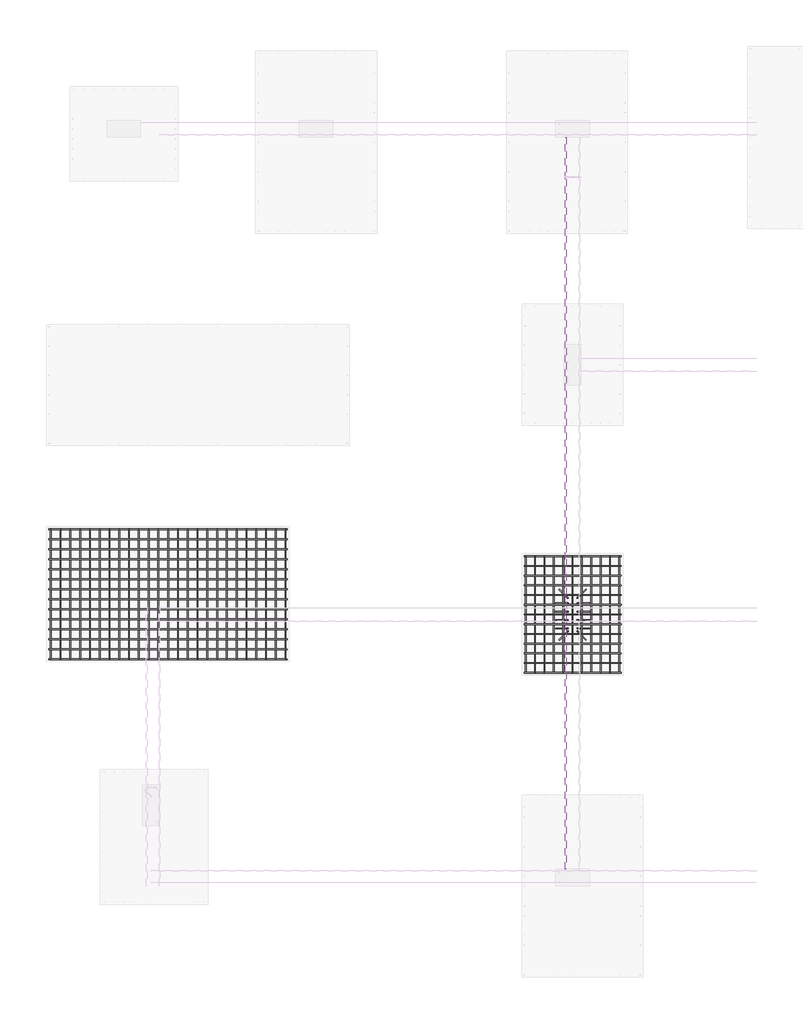
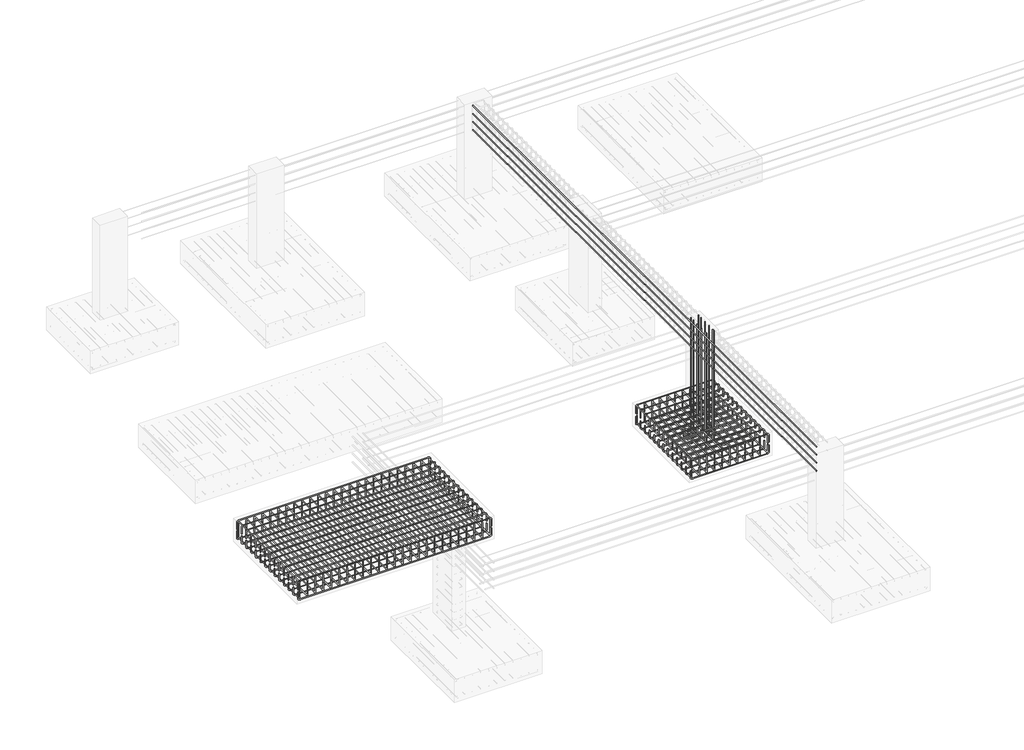
# One storey, part 3 of 16: 15 reinforcing bars.
"""IFC4 building model written with IfcOpenShell, lengths in millimetres."""

from ifc_helpers import new_model, si_unit, point, frame, origin, place, context, project, spatial, polyline, circle_curve, trimmed, segment, composite_curve, source, transform, mapped, element, save
from ifc_brep_helpers import swept_disk

model = new_model("IFC4")

# Units and contexts
model_context = context("Model", 3, world=origin())
ifc_project = project(units=[si_unit("LENGTHUNIT", "METRE", prefix="MILLI")], contexts=[model_context])

# Site, building, storey
site = spatial("IfcSite", under=ifc_project)
building = spatial("IfcBuilding", under=site)
storey = spatial("IfcBuildingStorey", under=building, Elevation=-1828.8)

# Reinforcing bars
placement = place(None, origin())
reinforcing_bar_shape = source(origin(), model_context, "Body", "SolidModel", [
    swept_disk(composite_curve([segment(polyline([(-8214.2725801, -1513.6888221, -2088.8), (-8214.2725801, -1513.6888221, -2212.8)]), True, "CONTINUOUS"), segment(trimmed(circle_curve(frame((-8244.2725801, -1513.6888221, -2212.8), z_axis=(0.0, 1.0, 0.0), x_axis=(30.0, 0.0, 0.0)), 30.0), [point((-8214.2725801, -1513.6888221, -2212.8))], [point((-8244.2725801, -1513.6888221, -2242.8))], True, "CARTESIAN"), True, "CONTINUOUS"), segment(polyline([(-8244.2725801, -1513.6888221, -2242.8), (-9612.2725801, -1513.6888221, -2242.8)]), True, "CONTINUOUS"), segment(trimmed(circle_curve(frame((-9612.2725801, -1513.6888221, -2212.8), z_axis=(0.0, 1.0, 0.0), x_axis=(0.0, 0.0, -30.0)), 30.0), [point((-9612.2725801, -1513.6888221, -2242.8))], [point((-9642.2725801, -1513.6888221, -2212.8))], True, "CARTESIAN"), True, "CONTINUOUS"), segment(polyline([(-9642.2725801, -1513.6888221, -2212.8), (-9642.2725801, -1513.6888221, -2088.8)]), True, "CONTINUOUS")], self_intersect=False), 6.0),
])
element("IfcReinforcingBar", 1, at=placement, inside=storey, context=model_context, shape_type="MappedRepresentation", body=[
    mapped(reinforcing_bar_shape, transform((0.0, 0.0, 0.0), x_axis=(1.0, 0.0, 0.0), y_axis=(0.0, 1.0, 0.0), z_axis=(0.0, 0.0, 1.0))),
    mapped(reinforcing_bar_shape, transform((0.0, -144.0, 0.0), x_axis=(1.0, 0.0, 0.0), y_axis=(0.0, 1.0, 0.0), z_axis=(0.0, 0.0, 1.0))),
    mapped(reinforcing_bar_shape, transform((0.0, -288.0, 0.0), x_axis=(1.0, 0.0, 0.0), y_axis=(0.0, 1.0, 0.0), z_axis=(0.0, 0.0, 1.0))),
    mapped(reinforcing_bar_shape, transform((0.0, -432.0, 0.0), x_axis=(1.0, 0.0, 0.0), y_axis=(0.0, 1.0, 0.0), z_axis=(0.0, 0.0, 1.0))),
    mapped(reinforcing_bar_shape, transform((0.0, -576.0, 0.0), x_axis=(1.0, 0.0, 0.0), y_axis=(0.0, 1.0, 0.0), z_axis=(0.0, 0.0, 1.0))),
    mapped(reinforcing_bar_shape, transform((0.0, -720.0, 0.0), x_axis=(1.0, 0.0, 0.0), y_axis=(0.0, 1.0, 0.0), z_axis=(0.0, 0.0, 1.0))),
    mapped(reinforcing_bar_shape, transform((0.0, -864.0, 0.0), x_axis=(1.0, 0.0, 0.0), y_axis=(0.0, 1.0, 0.0), z_axis=(0.0, 0.0, 1.0))),
    mapped(reinforcing_bar_shape, transform((0.0, -1008.0, 0.0), x_axis=(1.0, 0.0, 0.0), y_axis=(0.0, 1.0, 0.0), z_axis=(0.0, 0.0, 1.0))),
    mapped(reinforcing_bar_shape, transform((0.0, -1152.0, 0.0), x_axis=(1.0, 0.0, 0.0), y_axis=(0.0, 1.0, 0.0), z_axis=(0.0, 0.0, 1.0))),
    mapped(reinforcing_bar_shape, transform((0.0, -1296.0, 0.0), x_axis=(1.0, 0.0, 0.0), y_axis=(0.0, 1.0, 0.0), z_axis=(0.0, 0.0, 1.0))),
    mapped(reinforcing_bar_shape, transform((0.0, -1440.0, 0.0), x_axis=(1.0, 0.0, 0.0), y_axis=(0.0, 1.0, 0.0), z_axis=(0.0, 0.0, 1.0))),
    mapped(reinforcing_bar_shape, transform((0.0, -1584.0, 0.0), x_axis=(1.0, 0.0, 0.0), y_axis=(0.0, 1.0, 0.0), z_axis=(0.0, 0.0, 1.0))),
    mapped(reinforcing_bar_shape, transform((0.0, -1728.0, 0.0), x_axis=(1.0, 0.0, 0.0), y_axis=(0.0, 1.0, 0.0), z_axis=(0.0, 0.0, 1.0))),
])
reinforcing_bar_2_shape = source(origin(), model_context, "Body", "SolidModel", [
    swept_disk(composite_curve([segment(polyline([(-9642.2725801, -1513.6888221, -2018.8), (-9642.2725801, -1513.6888221, -1894.8)]), True, "CONTINUOUS"), segment(trimmed(circle_curve(frame((-9612.2725801, -1513.6888221, -1894.8), z_axis=(0.0, 1.0, 0.0), x_axis=(-30.0, 0.0, 0.0)), 30.0), [point((-9642.2725801, -1513.6888221, -1894.8))], [point((-9612.2725801, -1513.6888221, -1864.8))], True, "CARTESIAN"), True, "CONTINUOUS"), segment(polyline([(-9612.2725801, -1513.6888221, -1864.8), (-8244.2725801, -1513.6888221, -1864.8)]), True, "CONTINUOUS"), segment(trimmed(circle_curve(frame((-8244.2725801, -1513.6888221, -1894.8), z_axis=(0.0, 1.0, 0.0), x_axis=(0.0, 0.0, 30.0)), 30.0), [point((-8244.2725801, -1513.6888221, -1864.8))], [point((-8214.2725801, -1513.6888221, -1894.8))], True, "CARTESIAN"), True, "CONTINUOUS"), segment(polyline([(-8214.2725801, -1513.6888221, -1894.8), (-8214.2725801, -1513.6888221, -2018.8)]), True, "CONTINUOUS")], self_intersect=False), 6.0),
])
element("IfcReinforcingBar", 2, at=placement, inside=storey, context=model_context, shape_type="MappedRepresentation", body=[
    mapped(reinforcing_bar_2_shape, transform((0.0, 0.0, 0.0), x_axis=(1.0, 0.0, 0.0), y_axis=(0.0, 1.0, 0.0), z_axis=(0.0, 0.0, 1.0))),
    mapped(reinforcing_bar_2_shape, transform((0.0, -144.0, 0.0), x_axis=(1.0, 0.0, 0.0), y_axis=(0.0, 1.0, 0.0), z_axis=(0.0, 0.0, 1.0))),
    mapped(reinforcing_bar_2_shape, transform((0.0, -288.0, 0.0), x_axis=(1.0, 0.0, 0.0), y_axis=(0.0, 1.0, 0.0), z_axis=(0.0, 0.0, 1.0))),
    mapped(reinforcing_bar_2_shape, transform((0.0, -432.0, 0.0), x_axis=(1.0, 0.0, 0.0), y_axis=(0.0, 1.0, 0.0), z_axis=(0.0, 0.0, 1.0))),
    mapped(reinforcing_bar_2_shape, transform((0.0, -576.0, 0.0), x_axis=(1.0, 0.0, 0.0), y_axis=(0.0, 1.0, 0.0), z_axis=(0.0, 0.0, 1.0))),
    mapped(reinforcing_bar_2_shape, transform((0.0, -720.0, 0.0), x_axis=(1.0, 0.0, 0.0), y_axis=(0.0, 1.0, 0.0), z_axis=(0.0, 0.0, 1.0))),
    mapped(reinforcing_bar_2_shape, transform((0.0, -864.0, 0.0), x_axis=(1.0, 0.0, 0.0), y_axis=(0.0, 1.0, 0.0), z_axis=(0.0, 0.0, 1.0))),
    mapped(reinforcing_bar_2_shape, transform((0.0, -1008.0, 0.0), x_axis=(1.0, 0.0, 0.0), y_axis=(0.0, 1.0, 0.0), z_axis=(0.0, 0.0, 1.0))),
    mapped(reinforcing_bar_2_shape, transform((0.0, -1152.0, 0.0), x_axis=(1.0, 0.0, 0.0), y_axis=(0.0, 1.0, 0.0), z_axis=(0.0, 0.0, 1.0))),
    mapped(reinforcing_bar_2_shape, transform((0.0, -1296.0, 0.0), x_axis=(1.0, 0.0, 0.0), y_axis=(0.0, 1.0, 0.0), z_axis=(0.0, 0.0, 1.0))),
    mapped(reinforcing_bar_2_shape, transform((0.0, -1440.0, 0.0), x_axis=(1.0, 0.0, 0.0), y_axis=(0.0, 1.0, 0.0), z_axis=(0.0, 0.0, 1.0))),
    mapped(reinforcing_bar_2_shape, transform((0.0, -1584.0, 0.0), x_axis=(1.0, 0.0, 0.0), y_axis=(0.0, 1.0, 0.0), z_axis=(0.0, 0.0, 1.0))),
    mapped(reinforcing_bar_2_shape, transform((0.0, -1728.0, 0.0), x_axis=(1.0, 0.0, 0.0), y_axis=(0.0, 1.0, 0.0), z_axis=(0.0, 0.0, 1.0))),
])
reinforcing_bar_3_shape = source(origin(), model_context, "Body", "SolidModel", [
    swept_disk(composite_curve([segment(polyline([(-9625.0397909, -1513.6888221, -2072.0951729), (-9625.0397909, -1513.6888221, -2196.0951729)]), True, "CONTINUOUS"), segment(trimmed(circle_curve(frame((-9625.0397909, -1543.6888221, -2196.0951729), z_axis=(-1.0, 0.0, 0.0), x_axis=(0.0, 30.0, 0.0)), 30.0), [point((-9625.0397909, -1513.6888221, -2196.0951729))], [point((-9625.0397909, -1543.6888221, -2226.0951729))], True, "CARTESIAN"), True, "CONTINUOUS"), segment(polyline([(-9625.0397909, -1543.6888221, -2226.0951729), (-9625.0397909, -3211.6888221, -2226.0951729)]), True, "CONTINUOUS"), segment(trimmed(circle_curve(frame((-9625.0397909, -3211.6888221, -2196.0951729), z_axis=(-1.0, 0.0, 0.0), x_axis=(0.0, 0.0, -30.0)), 30.0), [point((-9625.0397909, -3211.6888221, -2226.0951729))], [point((-9625.0397909, -3241.6888221, -2196.0951729))], True, "CARTESIAN"), True, "CONTINUOUS"), segment(polyline([(-9625.0397909, -3241.6888221, -2196.0951729), (-9625.0397909, -3241.6888221, -2072.0951729)]), True, "CONTINUOUS")], self_intersect=False), 6.0),
])
element("IfcReinforcingBar", 3, at=placement, inside=storey, context=model_context, shape_type="MappedRepresentation", body=[
    mapped(reinforcing_bar_3_shape, transform((0.0, 0.0, 0.0), x_axis=(1.0, 0.0, 0.0), y_axis=(0.0, 1.0, 0.0), z_axis=(0.0, 0.0, 1.0))),
    mapped(reinforcing_bar_3_shape, transform((138.8820351, 0.0, 0.0), x_axis=(1.0, 0.0, 0.0), y_axis=(0.0, 1.0, 0.0), z_axis=(0.0, 0.0, 1.0))),
    mapped(reinforcing_bar_3_shape, transform((277.7640703, 0.0, 0.0), x_axis=(1.0, 0.0, 0.0), y_axis=(0.0, 1.0, 0.0), z_axis=(0.0, 0.0, 1.0))),
    mapped(reinforcing_bar_3_shape, transform((416.6461054, 0.0, 0.0), x_axis=(1.0, 0.0, 0.0), y_axis=(0.0, 1.0, 0.0), z_axis=(0.0, 0.0, 1.0))),
    mapped(reinforcing_bar_3_shape, transform((555.5281406, 0.0, 0.0), x_axis=(1.0, 0.0, 0.0), y_axis=(0.0, 1.0, 0.0), z_axis=(0.0, 0.0, 1.0))),
    mapped(reinforcing_bar_3_shape, transform((694.4101757, 0.0, 0.0), x_axis=(1.0, 0.0, 0.0), y_axis=(0.0, 1.0, 0.0), z_axis=(0.0, 0.0, 1.0))),
    mapped(reinforcing_bar_3_shape, transform((833.2922109, 0.0, 0.0), x_axis=(1.0, 0.0, 0.0), y_axis=(0.0, 1.0, 0.0), z_axis=(0.0, 0.0, 1.0))),
    mapped(reinforcing_bar_3_shape, transform((972.174246, 0.0, 0.0), x_axis=(1.0, 0.0, 0.0), y_axis=(0.0, 1.0, 0.0), z_axis=(0.0, 0.0, 1.0))),
    mapped(reinforcing_bar_3_shape, transform((1111.0562811, 0.0, 0.0), x_axis=(1.0, 0.0, 0.0), y_axis=(0.0, 1.0, 0.0), z_axis=(0.0, 0.0, 1.0))),
    mapped(reinforcing_bar_3_shape, transform((1249.9383163, 0.0, 0.0), x_axis=(1.0, 0.0, 0.0), y_axis=(0.0, 1.0, 0.0), z_axis=(0.0, 0.0, 1.0))),
    mapped(reinforcing_bar_3_shape, transform((1388.8203514, 0.0, 0.0), x_axis=(1.0, 0.0, 0.0), y_axis=(0.0, 1.0, 0.0), z_axis=(0.0, 0.0, 1.0))),
])
reinforcing_bar_4_shape = source(origin(), model_context, "Body", "SolidModel", [
    swept_disk(composite_curve([segment(polyline([(-8236.2194394, -1513.6888221, -2034.1277079), (-8236.2194394, -1513.6888221, -1910.1277079)]), True, "CONTINUOUS"), segment(trimmed(circle_curve(frame((-8236.2194394, -1543.6888221, -1910.1277079), z_axis=(1.0, 0.0, 0.0), x_axis=(0.0, 30.0, 0.0)), 30.0), [point((-8236.2194394, -1513.6888221, -1910.1277079))], [point((-8236.2194394, -1543.6888221, -1880.1277079))], True, "CARTESIAN"), True, "CONTINUOUS"), segment(polyline([(-8236.2194394, -1543.6888221, -1880.1277079), (-8236.2194394, -3211.6888221, -1880.1277079)]), True, "CONTINUOUS"), segment(trimmed(circle_curve(frame((-8236.2194394, -3211.6888221, -1910.1277079), z_axis=(1.0, 0.0, 0.0), x_axis=(0.0, 0.0, 30.0)), 30.0), [point((-8236.2194394, -3211.6888221, -1880.1277079))], [point((-8236.2194394, -3241.6888221, -1910.1277079))], True, "CARTESIAN"), True, "CONTINUOUS"), segment(polyline([(-8236.2194394, -3241.6888221, -1910.1277079), (-8236.2194394, -3241.6888221, -2034.1277079)]), True, "CONTINUOUS")], self_intersect=False), 6.0),
])
element("IfcReinforcingBar", 4, at=placement, inside=storey, context=model_context, shape_type="MappedRepresentation", body=[
    mapped(reinforcing_bar_4_shape, transform((0.0, 0.0, 0.0), x_axis=(1.0, 0.0, 0.0), y_axis=(0.0, 1.0, 0.0), z_axis=(0.0, 0.0, 1.0))),
    mapped(reinforcing_bar_4_shape, transform((-138.8820351, 0.0, 0.0), x_axis=(1.0, 0.0, 0.0), y_axis=(0.0, 1.0, 0.0), z_axis=(0.0, 0.0, 1.0))),
    mapped(reinforcing_bar_4_shape, transform((-277.7640703, 0.0, 0.0), x_axis=(1.0, 0.0, 0.0), y_axis=(0.0, 1.0, 0.0), z_axis=(0.0, 0.0, 1.0))),
    mapped(reinforcing_bar_4_shape, transform((-416.6461054, 0.0, 0.0), x_axis=(1.0, 0.0, 0.0), y_axis=(0.0, 1.0, 0.0), z_axis=(0.0, 0.0, 1.0))),
    mapped(reinforcing_bar_4_shape, transform((-555.5281406, 0.0, 0.0), x_axis=(1.0, 0.0, 0.0), y_axis=(0.0, 1.0, 0.0), z_axis=(0.0, 0.0, 1.0))),
    mapped(reinforcing_bar_4_shape, transform((-694.4101757, 0.0, 0.0), x_axis=(1.0, 0.0, 0.0), y_axis=(0.0, 1.0, 0.0), z_axis=(0.0, 0.0, 1.0))),
    mapped(reinforcing_bar_4_shape, transform((-833.2922109, 0.0, 0.0), x_axis=(1.0, 0.0, 0.0), y_axis=(0.0, 1.0, 0.0), z_axis=(0.0, 0.0, 1.0))),
    mapped(reinforcing_bar_4_shape, transform((-972.174246, 0.0, 0.0), x_axis=(1.0, 0.0, 0.0), y_axis=(0.0, 1.0, 0.0), z_axis=(0.0, 0.0, 1.0))),
    mapped(reinforcing_bar_4_shape, transform((-1111.0562811, 0.0, 0.0), x_axis=(1.0, 0.0, 0.0), y_axis=(0.0, 1.0, 0.0), z_axis=(0.0, 0.0, 1.0))),
    mapped(reinforcing_bar_4_shape, transform((-1249.9383163, 0.0, 0.0), x_axis=(1.0, 0.0, 0.0), y_axis=(0.0, 1.0, 0.0), z_axis=(0.0, 0.0, 1.0))),
    mapped(reinforcing_bar_4_shape, transform((-1388.8203514, 0.0, 0.0), x_axis=(1.0, 0.0, 0.0), y_axis=(0.0, 1.0, 0.0), z_axis=(0.0, 0.0, 1.0))),
])
reinforcing_bar_5_shape = source(origin(), model_context, "Body", "SolidModel", [
    swept_disk(composite_curve([segment(polyline([(-13164.3116599, -1115.1308991, -2072.7646888), (-13164.3116599, -1115.1308991, -2196.7646888)]), True, "CONTINUOUS"), segment(trimmed(circle_curve(frame((-13194.3116599, -1115.1308991, -2196.7646888), z_axis=(0.0, 1.0, 0.0), x_axis=(30.0, 0.0, 0.0)), 30.0), [point((-13164.3116599, -1115.1308991, -2196.7646888))], [point((-13194.3116599, -1115.1308991, -2226.7646888))], True, "CARTESIAN"), True, "CONTINUOUS"), segment(polyline([(-13194.3116599, -1115.1308991, -2226.7646888), (-16662.3116599, -1115.1308991, -2226.7646888)]), True, "CONTINUOUS"), segment(trimmed(circle_curve(frame((-16662.3116599, -1115.1308991, -2196.7646888), z_axis=(0.0, 1.0, 0.0), x_axis=(0.0, 0.0, -30.0)), 30.0), [point((-16662.3116599, -1115.1308991, -2226.7646888))], [point((-16692.3116599, -1115.1308991, -2196.7646888))], True, "CARTESIAN"), True, "CONTINUOUS"), segment(polyline([(-16692.3116599, -1115.1308991, -2196.7646888), (-16692.3116599, -1115.1308991, -2072.7646888)]), True, "CONTINUOUS")], self_intersect=False), 6.0),
])
element("IfcReinforcingBar", 5, at=placement, inside=storey, context=model_context, shape_type="MappedRepresentation", body=[
    mapped(reinforcing_bar_5_shape, transform((0.0, 0.0, 0.0), x_axis=(1.0, 0.0, 0.0), y_axis=(0.0, 1.0, 0.0), z_axis=(0.0, 0.0, 1.0))),
    mapped(reinforcing_bar_5_shape, transform((0.0, -148.3076923, 0.0), x_axis=(1.0, 0.0, 0.0), y_axis=(0.0, 1.0, 0.0), z_axis=(0.0, 0.0, 1.0))),
    mapped(reinforcing_bar_5_shape, transform((0.0, -296.6153846, 0.0), x_axis=(1.0, 0.0, 0.0), y_axis=(0.0, 1.0, 0.0), z_axis=(0.0, 0.0, 1.0))),
    mapped(reinforcing_bar_5_shape, transform((0.0, -444.9230769, 0.0), x_axis=(1.0, 0.0, 0.0), y_axis=(0.0, 1.0, 0.0), z_axis=(0.0, 0.0, 1.0))),
    mapped(reinforcing_bar_5_shape, transform((0.0, -593.2307692, 0.0), x_axis=(1.0, 0.0, 0.0), y_axis=(0.0, 1.0, 0.0), z_axis=(0.0, 0.0, 1.0))),
    mapped(reinforcing_bar_5_shape, transform((0.0, -741.5384615, 0.0), x_axis=(1.0, 0.0, 0.0), y_axis=(0.0, 1.0, 0.0), z_axis=(0.0, 0.0, 1.0))),
    mapped(reinforcing_bar_5_shape, transform((0.0, -889.8461538, 0.0), x_axis=(1.0, 0.0, 0.0), y_axis=(0.0, 1.0, 0.0), z_axis=(0.0, 0.0, 1.0))),
    mapped(reinforcing_bar_5_shape, transform((0.0, -1038.1538462, 0.0), x_axis=(1.0, 0.0, 0.0), y_axis=(0.0, 1.0, 0.0), z_axis=(0.0, 0.0, 1.0))),
    mapped(reinforcing_bar_5_shape, transform((0.0, -1186.4615385, 0.0), x_axis=(1.0, 0.0, 0.0), y_axis=(0.0, 1.0, 0.0), z_axis=(0.0, 0.0, 1.0))),
    mapped(reinforcing_bar_5_shape, transform((0.0, -1334.7692308, 0.0), x_axis=(1.0, 0.0, 0.0), y_axis=(0.0, 1.0, 0.0), z_axis=(0.0, 0.0, 1.0))),
    mapped(reinforcing_bar_5_shape, transform((0.0, -1483.0769231, 0.0), x_axis=(1.0, 0.0, 0.0), y_axis=(0.0, 1.0, 0.0), z_axis=(0.0, 0.0, 1.0))),
    mapped(reinforcing_bar_5_shape, transform((0.0, -1631.3846154, 0.0), x_axis=(1.0, 0.0, 0.0), y_axis=(0.0, 1.0, 0.0), z_axis=(0.0, 0.0, 1.0))),
    mapped(reinforcing_bar_5_shape, transform((0.0, -1779.6923077, 0.0), x_axis=(1.0, 0.0, 0.0), y_axis=(0.0, 1.0, 0.0), z_axis=(0.0, 0.0, 1.0))),
    mapped(reinforcing_bar_5_shape, transform((0.0, -1928.0, 0.0), x_axis=(1.0, 0.0, 0.0), y_axis=(0.0, 1.0, 0.0), z_axis=(0.0, 0.0, 1.0))),
])
reinforcing_bar_6_shape = source(origin(), model_context, "Body", "SolidModel", [
    swept_disk(composite_curve([segment(polyline([(-16692.3116599, -1115.1308991, -2026.8886474), (-16692.3116599, -1115.1308991, -1902.8886474)]), True, "CONTINUOUS"), segment(trimmed(circle_curve(frame((-16662.3116599, -1115.1308991, -1902.8886474), z_axis=(0.0, 1.0, 0.0), x_axis=(-30.0, 0.0, 0.0)), 30.0), [point((-16692.3116599, -1115.1308991, -1902.8886474))], [point((-16662.3116599, -1115.1308991, -1872.8886474))], True, "CARTESIAN"), True, "CONTINUOUS"), segment(polyline([(-16662.3116599, -1115.1308991, -1872.8886474), (-13194.3116599, -1115.1308991, -1872.8886474)]), True, "CONTINUOUS"), segment(trimmed(circle_curve(frame((-13194.3116599, -1115.1308991, -1902.8886474), z_axis=(0.0, 1.0, 0.0), x_axis=(0.0, 0.0, 30.0)), 30.0), [point((-13194.3116599, -1115.1308991, -1872.8886474))], [point((-13164.3116599, -1115.1308991, -1902.8886474))], True, "CARTESIAN"), True, "CONTINUOUS"), segment(polyline([(-13164.3116599, -1115.1308991, -1902.8886474), (-13164.3116599, -1115.1308991, -2026.8886474)]), True, "CONTINUOUS")], self_intersect=False), 6.0),
])
element("IfcReinforcingBar", 6, at=placement, inside=storey, context=model_context, shape_type="MappedRepresentation", body=[
    mapped(reinforcing_bar_6_shape, transform((0.0, 0.0, 0.0), x_axis=(1.0, 0.0, 0.0), y_axis=(0.0, 1.0, 0.0), z_axis=(0.0, 0.0, 1.0))),
    mapped(reinforcing_bar_6_shape, transform((0.0, -148.3076923, 0.0), x_axis=(1.0, 0.0, 0.0), y_axis=(0.0, 1.0, 0.0), z_axis=(0.0, 0.0, 1.0))),
    mapped(reinforcing_bar_6_shape, transform((0.0, -296.6153846, 0.0), x_axis=(1.0, 0.0, 0.0), y_axis=(0.0, 1.0, 0.0), z_axis=(0.0, 0.0, 1.0))),
    mapped(reinforcing_bar_6_shape, transform((0.0, -444.9230769, 0.0), x_axis=(1.0, 0.0, 0.0), y_axis=(0.0, 1.0, 0.0), z_axis=(0.0, 0.0, 1.0))),
    mapped(reinforcing_bar_6_shape, transform((0.0, -593.2307692, 0.0), x_axis=(1.0, 0.0, 0.0), y_axis=(0.0, 1.0, 0.0), z_axis=(0.0, 0.0, 1.0))),
    mapped(reinforcing_bar_6_shape, transform((0.0, -741.5384615, 0.0), x_axis=(1.0, 0.0, 0.0), y_axis=(0.0, 1.0, 0.0), z_axis=(0.0, 0.0, 1.0))),
    mapped(reinforcing_bar_6_shape, transform((0.0, -889.8461538, 0.0), x_axis=(1.0, 0.0, 0.0), y_axis=(0.0, 1.0, 0.0), z_axis=(0.0, 0.0, 1.0))),
    mapped(reinforcing_bar_6_shape, transform((0.0, -1038.1538462, 0.0), x_axis=(1.0, 0.0, 0.0), y_axis=(0.0, 1.0, 0.0), z_axis=(0.0, 0.0, 1.0))),
    mapped(reinforcing_bar_6_shape, transform((0.0, -1186.4615385, 0.0), x_axis=(1.0, 0.0, 0.0), y_axis=(0.0, 1.0, 0.0), z_axis=(0.0, 0.0, 1.0))),
    mapped(reinforcing_bar_6_shape, transform((0.0, -1334.7692308, 0.0), x_axis=(1.0, 0.0, 0.0), y_axis=(0.0, 1.0, 0.0), z_axis=(0.0, 0.0, 1.0))),
    mapped(reinforcing_bar_6_shape, transform((0.0, -1483.0769231, 0.0), x_axis=(1.0, 0.0, 0.0), y_axis=(0.0, 1.0, 0.0), z_axis=(0.0, 0.0, 1.0))),
    mapped(reinforcing_bar_6_shape, transform((0.0, -1631.3846154, 0.0), x_axis=(1.0, 0.0, 0.0), y_axis=(0.0, 1.0, 0.0), z_axis=(0.0, 0.0, 1.0))),
    mapped(reinforcing_bar_6_shape, transform((0.0, -1779.6923077, 0.0), x_axis=(1.0, 0.0, 0.0), y_axis=(0.0, 1.0, 0.0), z_axis=(0.0, 0.0, 1.0))),
    mapped(reinforcing_bar_6_shape, transform((0.0, -1928.0, 0.0), x_axis=(1.0, 0.0, 0.0), y_axis=(0.0, 1.0, 0.0), z_axis=(0.0, 0.0, 1.0))),
])
reinforcing_bar_7_shape = source(origin(), model_context, "Body", "SolidModel", [
    swept_disk(composite_curve([segment(polyline([(-16665.3962792, -1115.1308991, -2055.302566), (-16665.3962792, -1115.1308991, -2179.302566)]), True, "CONTINUOUS"), segment(trimmed(circle_curve(frame((-16665.3962792, -1145.1308991, -2179.302566), z_axis=(-1.0, 0.0, 0.0), x_axis=(0.0, 30.0, 0.0)), 30.0), [point((-16665.3962792, -1115.1308991, -2179.302566))], [point((-16665.3962792, -1145.1308991, -2209.302566))], True, "CARTESIAN"), True, "CONTINUOUS"), segment(polyline([(-16665.3962792, -1145.1308991, -2209.302566), (-16665.3962792, -3013.1308991, -2209.302566)]), True, "CONTINUOUS"), segment(trimmed(circle_curve(frame((-16665.3962792, -3013.1308991, -2179.302566), z_axis=(-1.0, 0.0, 0.0), x_axis=(0.0, 0.0, -30.0)), 30.0), [point((-16665.3962792, -3013.1308991, -2209.302566))], [point((-16665.3962792, -3043.1308991, -2179.302566))], True, "CARTESIAN"), True, "CONTINUOUS"), segment(polyline([(-16665.3962792, -3043.1308991, -2179.302566), (-16665.3962792, -3043.1308991, -2055.302566)]), True, "CONTINUOUS")], self_intersect=False), 6.0),
])
element("IfcReinforcingBar", 7, at=placement, inside=storey, context=model_context, shape_type="MappedRepresentation", body=[
    mapped(reinforcing_bar_7_shape, transform((0.0, 0.0, 0.0), x_axis=(1.0, 0.0, 0.0), y_axis=(0.0, 1.0, 0.0), z_axis=(0.0, 0.0, 1.0))),
    mapped(reinforcing_bar_7_shape, transform((145.0375224, 0.0, 0.0), x_axis=(1.0, 0.0, 0.0), y_axis=(0.0, 1.0, 0.0), z_axis=(0.0, 0.0, 1.0))),
    mapped(reinforcing_bar_7_shape, transform((290.0750448, 0.0, 0.0), x_axis=(1.0, 0.0, 0.0), y_axis=(0.0, 1.0, 0.0), z_axis=(0.0, 0.0, 1.0))),
    mapped(reinforcing_bar_7_shape, transform((435.1125672, 0.0, 0.0), x_axis=(1.0, 0.0, 0.0), y_axis=(0.0, 1.0, 0.0), z_axis=(0.0, 0.0, 1.0))),
    mapped(reinforcing_bar_7_shape, transform((580.1500896, 0.0, 0.0), x_axis=(1.0, 0.0, 0.0), y_axis=(0.0, 1.0, 0.0), z_axis=(0.0, 0.0, 1.0))),
    mapped(reinforcing_bar_7_shape, transform((725.187612, 0.0, 0.0), x_axis=(1.0, 0.0, 0.0), y_axis=(0.0, 1.0, 0.0), z_axis=(0.0, 0.0, 1.0))),
    mapped(reinforcing_bar_7_shape, transform((870.2251345, 0.0, 0.0), x_axis=(1.0, 0.0, 0.0), y_axis=(0.0, 1.0, 0.0), z_axis=(0.0, 0.0, 1.0))),
    mapped(reinforcing_bar_7_shape, transform((1015.2626569, 0.0, 0.0), x_axis=(1.0, 0.0, 0.0), y_axis=(0.0, 1.0, 0.0), z_axis=(0.0, 0.0, 1.0))),
    mapped(reinforcing_bar_7_shape, transform((1160.3001793, 0.0, 0.0), x_axis=(1.0, 0.0, 0.0), y_axis=(0.0, 1.0, 0.0), z_axis=(0.0, 0.0, 1.0))),
    mapped(reinforcing_bar_7_shape, transform((1305.3377017, 0.0, 0.0), x_axis=(1.0, 0.0, 0.0), y_axis=(0.0, 1.0, 0.0), z_axis=(0.0, 0.0, 1.0))),
    mapped(reinforcing_bar_7_shape, transform((1450.3752241, 0.0, 0.0), x_axis=(1.0, 0.0, 0.0), y_axis=(0.0, 1.0, 0.0), z_axis=(0.0, 0.0, 1.0))),
    mapped(reinforcing_bar_7_shape, transform((1595.4127465, 0.0, 0.0), x_axis=(1.0, 0.0, 0.0), y_axis=(0.0, 1.0, 0.0), z_axis=(0.0, 0.0, 1.0))),
    mapped(reinforcing_bar_7_shape, transform((1740.4502689, 0.0, 0.0), x_axis=(1.0, 0.0, 0.0), y_axis=(0.0, 1.0, 0.0), z_axis=(0.0, 0.0, 1.0))),
    mapped(reinforcing_bar_7_shape, transform((1885.4877913, 0.0, 0.0), x_axis=(1.0, 0.0, 0.0), y_axis=(0.0, 1.0, 0.0), z_axis=(0.0, 0.0, 1.0))),
    mapped(reinforcing_bar_7_shape, transform((2030.5253137, 0.0, 0.0), x_axis=(1.0, 0.0, 0.0), y_axis=(0.0, 1.0, 0.0), z_axis=(0.0, 0.0, 1.0))),
    mapped(reinforcing_bar_7_shape, transform((2175.5628361, 0.0, 0.0), x_axis=(1.0, 0.0, 0.0), y_axis=(0.0, 1.0, 0.0), z_axis=(0.0, 0.0, 1.0))),
    mapped(reinforcing_bar_7_shape, transform((2320.6003586, 0.0, 0.0), x_axis=(1.0, 0.0, 0.0), y_axis=(0.0, 1.0, 0.0), z_axis=(0.0, 0.0, 1.0))),
    mapped(reinforcing_bar_7_shape, transform((2465.637881, 0.0, 0.0), x_axis=(1.0, 0.0, 0.0), y_axis=(0.0, 1.0, 0.0), z_axis=(0.0, 0.0, 1.0))),
    mapped(reinforcing_bar_7_shape, transform((2610.6754034, 0.0, 0.0), x_axis=(1.0, 0.0, 0.0), y_axis=(0.0, 1.0, 0.0), z_axis=(0.0, 0.0, 1.0))),
    mapped(reinforcing_bar_7_shape, transform((2755.7129258, 0.0, 0.0), x_axis=(1.0, 0.0, 0.0), y_axis=(0.0, 1.0, 0.0), z_axis=(0.0, 0.0, 1.0))),
    mapped(reinforcing_bar_7_shape, transform((2900.7504482, 0.0, 0.0), x_axis=(1.0, 0.0, 0.0), y_axis=(0.0, 1.0, 0.0), z_axis=(0.0, 0.0, 1.0))),
    mapped(reinforcing_bar_7_shape, transform((3045.7879706, 0.0, 0.0), x_axis=(1.0, 0.0, 0.0), y_axis=(0.0, 1.0, 0.0), z_axis=(0.0, 0.0, 1.0))),
    mapped(reinforcing_bar_7_shape, transform((3190.825493, 0.0, 0.0), x_axis=(1.0, 0.0, 0.0), y_axis=(0.0, 1.0, 0.0), z_axis=(0.0, 0.0, 1.0))),
    mapped(reinforcing_bar_7_shape, transform((3335.8630154, 0.0, 0.0), x_axis=(1.0, 0.0, 0.0), y_axis=(0.0, 1.0, 0.0), z_axis=(0.0, 0.0, 1.0))),
    mapped(reinforcing_bar_7_shape, transform((3480.9005378, 0.0, 0.0), x_axis=(1.0, 0.0, 0.0), y_axis=(0.0, 1.0, 0.0), z_axis=(0.0, 0.0, 1.0))),
])
reinforcing_bar_8_shape = source(origin(), model_context, "Body", "SolidModel", [
    swept_disk(composite_curve([segment(polyline([(-13184.4957413, -1115.1308991, -2042.2263024), (-13184.4957413, -1115.1308991, -1918.2263024)]), True, "CONTINUOUS"), segment(trimmed(circle_curve(frame((-13184.4957413, -1145.1308991, -1918.2263024), z_axis=(1.0, 0.0, 0.0), x_axis=(0.0, 30.0, 0.0)), 30.0), [point((-13184.4957413, -1115.1308991, -1918.2263024))], [point((-13184.4957413, -1145.1308991, -1888.2263024))], True, "CARTESIAN"), True, "CONTINUOUS"), segment(polyline([(-13184.4957413, -1145.1308991, -1888.2263024), (-13184.4957413, -3013.1308991, -1888.2263024)]), True, "CONTINUOUS"), segment(trimmed(circle_curve(frame((-13184.4957413, -3013.1308991, -1918.2263024), z_axis=(1.0, 0.0, 0.0), x_axis=(0.0, 0.0, 30.0)), 30.0), [point((-13184.4957413, -3013.1308991, -1888.2263024))], [point((-13184.4957413, -3043.1308991, -1918.2263024))], True, "CARTESIAN"), True, "CONTINUOUS"), segment(polyline([(-13184.4957413, -3043.1308991, -1918.2263024), (-13184.4957413, -3043.1308991, -2042.2263024)]), True, "CONTINUOUS")], self_intersect=False), 6.0),
])
element("IfcReinforcingBar", 8, at=placement, inside=storey, context=model_context, shape_type="MappedRepresentation", body=[
    mapped(reinforcing_bar_8_shape, transform((0.0, 0.0, 0.0), x_axis=(1.0, 0.0, 0.0), y_axis=(0.0, 1.0, 0.0), z_axis=(0.0, 0.0, 1.0))),
    mapped(reinforcing_bar_8_shape, transform((-145.0375224, 0.0, 0.0), x_axis=(1.0, 0.0, 0.0), y_axis=(0.0, 1.0, 0.0), z_axis=(0.0, 0.0, 1.0))),
    mapped(reinforcing_bar_8_shape, transform((-290.0750448, 0.0, 0.0), x_axis=(1.0, 0.0, 0.0), y_axis=(0.0, 1.0, 0.0), z_axis=(0.0, 0.0, 1.0))),
    mapped(reinforcing_bar_8_shape, transform((-435.1125672, 0.0, 0.0), x_axis=(1.0, 0.0, 0.0), y_axis=(0.0, 1.0, 0.0), z_axis=(0.0, 0.0, 1.0))),
    mapped(reinforcing_bar_8_shape, transform((-580.1500896, 0.0, 0.0), x_axis=(1.0, 0.0, 0.0), y_axis=(0.0, 1.0, 0.0), z_axis=(0.0, 0.0, 1.0))),
    mapped(reinforcing_bar_8_shape, transform((-725.187612, 0.0, 0.0), x_axis=(1.0, 0.0, 0.0), y_axis=(0.0, 1.0, 0.0), z_axis=(0.0, 0.0, 1.0))),
    mapped(reinforcing_bar_8_shape, transform((-870.2251345, 0.0, 0.0), x_axis=(1.0, 0.0, 0.0), y_axis=(0.0, 1.0, 0.0), z_axis=(0.0, 0.0, 1.0))),
    mapped(reinforcing_bar_8_shape, transform((-1015.2626569, 0.0, 0.0), x_axis=(1.0, 0.0, 0.0), y_axis=(0.0, 1.0, 0.0), z_axis=(0.0, 0.0, 1.0))),
    mapped(reinforcing_bar_8_shape, transform((-1160.3001793, 0.0, 0.0), x_axis=(1.0, 0.0, 0.0), y_axis=(0.0, 1.0, 0.0), z_axis=(0.0, 0.0, 1.0))),
    mapped(reinforcing_bar_8_shape, transform((-1305.3377017, 0.0, 0.0), x_axis=(1.0, 0.0, 0.0), y_axis=(0.0, 1.0, 0.0), z_axis=(0.0, 0.0, 1.0))),
    mapped(reinforcing_bar_8_shape, transform((-1450.3752241, 0.0, 0.0), x_axis=(1.0, 0.0, 0.0), y_axis=(0.0, 1.0, 0.0), z_axis=(0.0, 0.0, 1.0))),
    mapped(reinforcing_bar_8_shape, transform((-1595.4127465, 0.0, 0.0), x_axis=(1.0, 0.0, 0.0), y_axis=(0.0, 1.0, 0.0), z_axis=(0.0, 0.0, 1.0))),
    mapped(reinforcing_bar_8_shape, transform((-1740.4502689, 0.0, 0.0), x_axis=(1.0, 0.0, 0.0), y_axis=(0.0, 1.0, 0.0), z_axis=(0.0, 0.0, 1.0))),
    mapped(reinforcing_bar_8_shape, transform((-1885.4877913, 0.0, 0.0), x_axis=(1.0, 0.0, 0.0), y_axis=(0.0, 1.0, 0.0), z_axis=(0.0, 0.0, 1.0))),
    mapped(reinforcing_bar_8_shape, transform((-2030.5253137, 0.0, 0.0), x_axis=(1.0, 0.0, 0.0), y_axis=(0.0, 1.0, 0.0), z_axis=(0.0, 0.0, 1.0))),
    mapped(reinforcing_bar_8_shape, transform((-2175.5628361, 0.0, 0.0), x_axis=(1.0, 0.0, 0.0), y_axis=(0.0, 1.0, 0.0), z_axis=(0.0, 0.0, 1.0))),
    mapped(reinforcing_bar_8_shape, transform((-2320.6003586, 0.0, 0.0), x_axis=(1.0, 0.0, 0.0), y_axis=(0.0, 1.0, 0.0), z_axis=(0.0, 0.0, 1.0))),
    mapped(reinforcing_bar_8_shape, transform((-2465.637881, 0.0, 0.0), x_axis=(1.0, 0.0, 0.0), y_axis=(0.0, 1.0, 0.0), z_axis=(0.0, 0.0, 1.0))),
    mapped(reinforcing_bar_8_shape, transform((-2610.6754034, 0.0, 0.0), x_axis=(1.0, 0.0, 0.0), y_axis=(0.0, 1.0, 0.0), z_axis=(0.0, 0.0, 1.0))),
    mapped(reinforcing_bar_8_shape, transform((-2755.7129258, 0.0, 0.0), x_axis=(1.0, 0.0, 0.0), y_axis=(0.0, 1.0, 0.0), z_axis=(0.0, 0.0, 1.0))),
    mapped(reinforcing_bar_8_shape, transform((-2900.7504482, 0.0, 0.0), x_axis=(1.0, 0.0, 0.0), y_axis=(0.0, 1.0, 0.0), z_axis=(0.0, 0.0, 1.0))),
    mapped(reinforcing_bar_8_shape, transform((-3045.7879706, 0.0, 0.0), x_axis=(1.0, 0.0, 0.0), y_axis=(0.0, 1.0, 0.0), z_axis=(0.0, 0.0, 1.0))),
    mapped(reinforcing_bar_8_shape, transform((-3190.825493, 0.0, 0.0), x_axis=(1.0, 0.0, 0.0), y_axis=(0.0, 1.0, 0.0), z_axis=(0.0, 0.0, 1.0))),
    mapped(reinforcing_bar_8_shape, transform((-3335.8630154, 0.0, 0.0), x_axis=(1.0, 0.0, 0.0), y_axis=(0.0, 1.0, 0.0), z_axis=(0.0, 0.0, 1.0))),
    mapped(reinforcing_bar_8_shape, transform((-3480.9005378, 0.0, 0.0), x_axis=(1.0, 0.0, 0.0), y_axis=(0.0, 1.0, 0.0), z_axis=(0.0, 0.0, 1.0))),
])
reinforcing_bar_9_shape = source(origin(), model_context, "Body", "SolidModel", [
    swept_disk(composite_curve([segment(polyline([(-8858.2317051, -2212.2776925, -30.0), (-8858.2317051, -2212.2776925, -2158.8)]), True, "CONTINUOUS"), segment(trimmed(circle_curve(frame((-8828.2317051, -2212.2776925, -2158.8), z_axis=(0.0, -1.0, 0.0), x_axis=(-30.0, 0.0, 0.0)), 30.0), [point((-8858.2317051, -2212.2776925, -2158.8))], [point((-8828.2317051, -2212.2776925, -2188.8))], True, "CARTESIAN"), True, "CONTINUOUS"), segment(polyline([(-8828.2317051, -2212.2776925, -2188.8), (-8675.8458602, -2212.2776925, -2188.8)]), True, "CONTINUOUS")], self_intersect=False), 6.0),
])
element("IfcReinforcingBar", 9, at=placement, inside=storey, context=model_context, shape_type="MappedRepresentation", body=[
    mapped(reinforcing_bar_9_shape, transform((0.0, 0.0, 0.0), x_axis=(1.0, 0.0, 0.0), y_axis=(0.0, 1.0, 0.0), z_axis=(0.0, 0.0, 1.0))),
    mapped(reinforcing_bar_9_shape, transform((0.0, -123.8384715, 0.0), x_axis=(1.0, 0.0, 0.0), y_axis=(0.0, 1.0, 0.0), z_axis=(0.0, 0.0, 1.0))),
    mapped(reinforcing_bar_9_shape, transform((0.0, -247.676943, 0.0), x_axis=(1.0, 0.0, 0.0), y_axis=(0.0, 1.0, 0.0), z_axis=(0.0, 0.0, 1.0))),
    mapped(reinforcing_bar_9_shape, transform((0.0, -371.5154145, 0.0), x_axis=(1.0, 0.0, 0.0), y_axis=(0.0, 1.0, 0.0), z_axis=(0.0, 0.0, 1.0))),
])
element("IfcReinforcingBar", 10, at=placement, inside=storey, context=model_context, shape_type="SolidModel", body=[
    swept_disk(composite_curve([segment(polyline([(-8998.3134551, -2134.0900242, -30.0), (-8998.3134551, -2134.0900242, -2158.8)]), True, "CONTINUOUS"), segment(trimmed(circle_curve(frame((-9019.5266585, -2112.8768207, -2158.8), z_axis=(0.7071067811865435, 0.7071067811865517, 0.0), x_axis=(21.213203400000566, -21.213203499999963, 0.0)), 30.0), [point((-8998.3134551, -2134.0900242, -2158.8))], [point((-9019.5266585, -2112.8768207, -2188.8))], True, "CARTESIAN"), True, "CONTINUOUS"), segment(polyline([(-9019.5266585, -2112.8768207, -2188.8), (-9127.2797228, -2005.1237565, -2188.8)]), True, "CONTINUOUS")], self_intersect=False), 6.0),
])
element("IfcReinforcingBar", 11, at=placement, inside=storey, context=model_context, shape_type="SolidModel", body=[
    swept_disk(composite_curve([segment(polyline([(-8858.2317051, -2624.1717741, -30.0), (-8858.2317051, -2624.1717741, -2158.8)]), True, "CONTINUOUS"), segment(trimmed(circle_curve(frame((-8837.0185017, -2645.3849776, -2158.8), z_axis=(-0.7071067811865435, -0.7071067811865517, 0.0), x_axis=(-21.213203400000566, 21.213203499999963, 0.0)), 30.0), [point((-8858.2317051, -2624.1717741, -2158.8))], [point((-8837.0185017, -2645.3849776, -2188.8))], True, "CARTESIAN"), True, "CONTINUOUS"), segment(polyline([(-8837.0185017, -2645.3849776, -2188.8), (-8729.2654374, -2753.1380418, -2188.8)]), True, "CONTINUOUS")], self_intersect=False), 6.0),
])
element("IfcReinforcingBar", 12, at=placement, inside=storey, context=model_context, shape_type="SolidModel", body=[
    swept_disk(composite_curve([segment(polyline([(-8998.3134551, -2624.1717741, -30.0), (-8998.3134551, -2624.1717741, -2158.8)]), True, "CONTINUOUS"), segment(trimmed(circle_curve(frame((-9019.5266585, -2645.3849776, -2158.8), z_axis=(-0.7071067811865435, 0.7071067811865516, 0.0), x_axis=(21.213203400000566, 21.213203499999963, 0.0)), 30.0), [point((-8998.3134551, -2624.1717741, -2158.8))], [point((-9019.5266585, -2645.3849776, -2188.8))], True, "CARTESIAN"), True, "CONTINUOUS"), segment(polyline([(-9019.5266585, -2645.3849776, -2188.8), (-9127.2797228, -2753.1380418, -2188.8)]), True, "CONTINUOUS")], self_intersect=False), 6.0),
])
element("IfcReinforcingBar", 13, at=placement, inside=storey, context=model_context, shape_type="SolidModel", body=[
    swept_disk(composite_curve([segment(polyline([(-8858.2317051, -2134.0900242, -30.0), (-8858.2317051, -2134.0900242, -2158.8)]), True, "CONTINUOUS"), segment(trimmed(circle_curve(frame((-8837.0185017, -2112.8768207, -2158.8), z_axis=(0.7071067811865434, -0.7071067811865518, 0.0), x_axis=(-21.213203400000566, -21.213203499999963, 0.0)), 30.0), [point((-8858.2317051, -2134.0900242, -2158.8))], [point((-8837.0185017, -2112.8768207, -2188.8))], True, "CARTESIAN"), True, "CONTINUOUS"), segment(polyline([(-8837.0185017, -2112.8768207, -2188.8), (-8729.2654374, -2005.1237565, -2188.8)]), True, "CONTINUOUS")], self_intersect=False), 6.0),
])
reinforcing_bar_10_shape = source(origin(), model_context, "Body", "SolidModel", [
    swept_disk(composite_curve([segment(polyline([(-8998.3134551, -2212.2776925, -30.0), (-8998.3134551, -2212.2776925, -2158.8)]), True, "CONTINUOUS"), segment(trimmed(circle_curve(frame((-9028.3134551, -2212.2776925, -2158.8), z_axis=(0.0, 1.0, 0.0), x_axis=(30.0, 0.0, 0.0)), 30.0), [point((-8998.3134551, -2212.2776925, -2158.8))], [point((-9028.3134551, -2212.2776925, -2188.8))], True, "CARTESIAN"), True, "CONTINUOUS"), segment(polyline([(-9028.3134551, -2212.2776925, -2188.8), (-9180.6992999, -2212.2776925, -2188.8)]), True, "CONTINUOUS")], self_intersect=False), 6.0),
])
element("IfcReinforcingBar", 14, at=placement, inside=storey, context=model_context, shape_type="MappedRepresentation", body=[
    mapped(reinforcing_bar_10_shape, transform((0.0, 0.0, 0.0), x_axis=(1.0, 0.0, 0.0), y_axis=(0.0, 1.0, 0.0), z_axis=(0.0, 0.0, 1.0))),
    mapped(reinforcing_bar_10_shape, transform((0.0, -123.8384715, 0.0), x_axis=(1.0, 0.0, 0.0), y_axis=(0.0, 1.0, 0.0), z_axis=(0.0, 0.0, 1.0))),
    mapped(reinforcing_bar_10_shape, transform((0.0, -247.676943, 0.0), x_axis=(1.0, 0.0, 0.0), y_axis=(0.0, 1.0, 0.0), z_axis=(0.0, 0.0, 1.0))),
    mapped(reinforcing_bar_10_shape, transform((0.0, -371.5154145, 0.0), x_axis=(1.0, 0.0, 0.0), y_axis=(0.0, 1.0, 0.0), z_axis=(0.0, 0.0, 1.0))),
])
reinforcing_bar_11_shape = source(origin(), model_context, "Body", "SolidModel", [
    swept_disk(composite_curve([segment(polyline([(-9030.2725801, 4699.6235223, -66.0), (-9030.2725801, -6152.9793469, -66.0)]), True, "CONTINUOUS")], self_intersect=False), 6.0),
])
element("IfcReinforcingBar", 15, at=placement, inside=storey, context=model_context, shape_type="MappedRepresentation", body=[
    mapped(reinforcing_bar_11_shape, transform((0.0, 0.0, 0.0), x_axis=(1.0, 0.0, 0.0), y_axis=(0.0, 1.0, 0.0), z_axis=(0.0, 0.0, 1.0))),
    mapped(reinforcing_bar_11_shape, transform((0.0, 0.0, -156.0), x_axis=(1.0, 0.0, 0.0), y_axis=(0.0, 1.0, 0.0), z_axis=(0.0, 0.0, 1.0))),
    mapped(reinforcing_bar_11_shape, transform((0.0, 0.0, -312.0), x_axis=(1.0, 0.0, 0.0), y_axis=(0.0, 1.0, 0.0), z_axis=(0.0, 0.0, 1.0))),
    mapped(reinforcing_bar_11_shape, transform((0.0, 0.0, -468.0), x_axis=(1.0, 0.0, 0.0), y_axis=(0.0, 1.0, 0.0), z_axis=(0.0, 0.0, 1.0))),
])

save(model, "model.ifc")

# Revit data of these elements
# Elements 1, 2, 3, 4, 5, 6, 7, 8, 9, 10, 11, 12, 13, 14, 15 (IfcReinforcingBar)
#   Phase Created = New Construction
